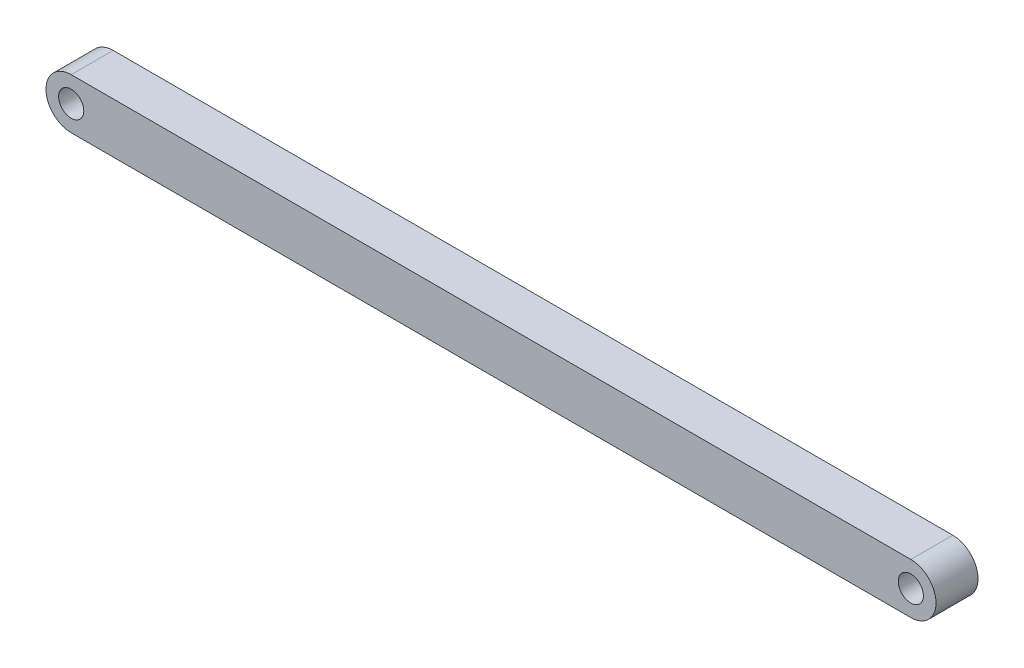
from build123d import *

# Parameters (mm, degrees)
LINK_PROFILE_SKETCH_R        = 1.5
LINK_BAR_100_CTRS_2X_3_DEPTH = 5


with BuildPart() as part:
    # Link Profile Sketch → Link Bar 100 Ctrs 2xØ3 (new body)
    with BuildSketch(Plane.XY):
        with BuildLine():
            Line((-50, 3), (50, 3))
            ThreePointArc((50, 3), (53, 0), (50, -3))
            Line((50, -3), (-50, -3))
            ThreePointArc((-50, -3), (-53, 0), (-50, 3))
        make_face()
        with Locations((-50, 0)):
            Circle(LINK_PROFILE_SKETCH_R, mode=Mode.SUBTRACT)
        with Locations((50, 0)):
            Circle(LINK_PROFILE_SKETCH_R, mode=Mode.SUBTRACT)
    extrude(amount=LINK_BAR_100_CTRS_2X_3_DEPTH)


solid = part.part
